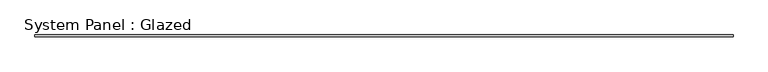
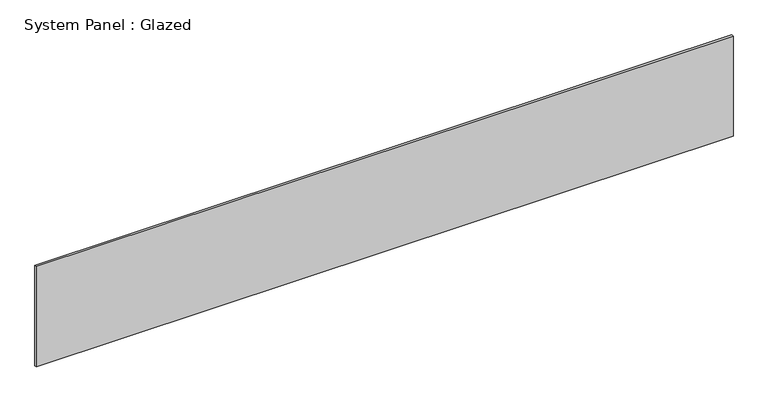
"""IFC4 building model written with IfcOpenShell, lengths in millimetres: plate geometry, System Panel : Glazed."""

from ifc_helpers import new_model, si_unit, origin, origin_with_axes, place, context, project, spatial, polyline, outline, extrude, source, transform, mapped, element, save


def system_panel_glazed_ae5726c8(model_context):
    return source(origin(), model_context, "Body", "SweptSolid", [
        extrude(outline(polyline([(4584.7, 19.05), (-4584.7, 19.05), (-4584.7, 44.45), (4584.7, 44.45), (4584.7, 19.05)])), origin_with_axes(), (0.0, 0.0, 1.0), 1397.0),
    ])


if __name__ == "__main__":
    model = new_model("IFC4")
    model_context = context("Model", 3, world=origin())
    ifc_project = project(units=[si_unit("LENGTHUNIT", "METRE", prefix="MILLI")], contexts=[model_context])
    site = spatial("IfcSite", under=ifc_project)
    building = spatial("IfcBuilding", under=site)
    placement = place(None, origin())
    system_panel_glazed_shape = system_panel_glazed_ae5726c8(model_context)
    element("IfcPlate", 1, ObjectType="System Panel : Glazed", at=placement, inside=building, context=model_context, shape_type="MappedRepresentation", body=[
        mapped(system_panel_glazed_shape, transform((0.0, 0.0, 0.0), x_axis=(1.0, 0.0, 0.0), y_axis=(0.0, 1.0, 0.0), z_axis=(0.0, 0.0, 1.0))),
    ])
    save(model, "model.ifc")

# Revit data of these elements
# Type "System Panel : Glazed"
#   Construction Type Id = "GSP4R"
#   Analytic Construction = "1/8 in Pilkington single glazing"
#   Visual Light Transmittance = 0.9
#   Solar Heat Gain Coefficient = 0.86
#   Heat Transfer Coefficient (U) = 1.18115 BTU/(h·ft²·°F)
# Element 1 (IfcPlate, "System Panel : Glazed")
#   Materials on its faces: "Glass"
# Materials
#   "Glass": class "Glass", colour RGB 0 128 192, transparency 0.75, Description = "Soda Lime Glass", Cost = 0
